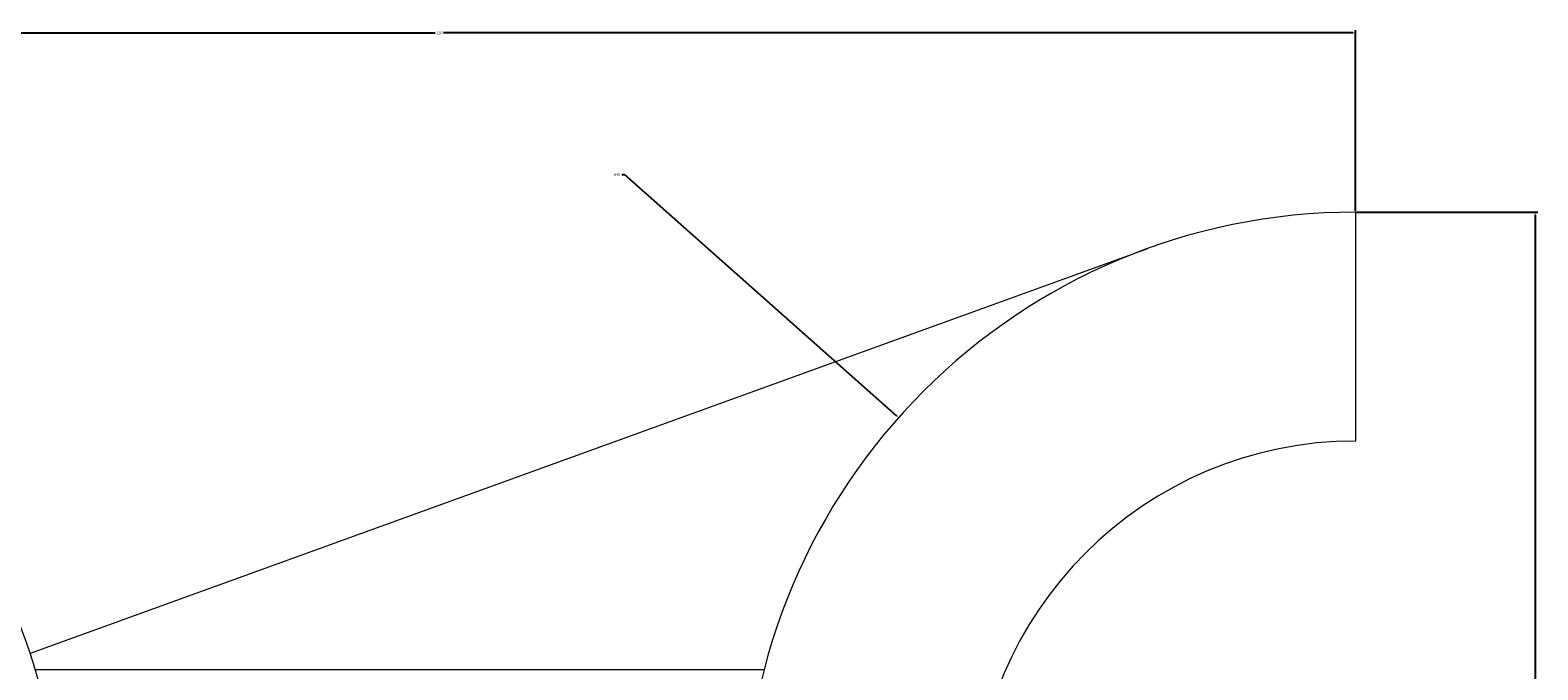
# Model space of a CAD drawing. Units: millimetres. Extents: x 3108 to 3332, y 1482 to 1586.
# Tile 5 of 5: x 3233 to 3332, y 1544 to 1586. Entities that reach past the tile are written whole.
import ezdxf

# ---------------------------------------------------------------- set-up
doc = ezdxf.new("R2010")
doc.units = ezdxf.units.MM
doc.layers.add('M-CONS', color=8, linetype='Continuous', lineweight=18)
doc.layers.add('M-DIMS', color=2, linetype='Continuous', lineweight=18)
doc.styles.get("Standard").update_dxf_attribs({"font": 'arial.ttf'})
doc.dimstyles.get("Standard").update_dxf_attribs({"dimtxt": 0.18, "dimasz": 0.18, "dimexe": 0.18, "dimexo": 0.0625, "dimgap": 0.09, "dimtad": 0, "dimtih": 1, "dimtoh": 1, "dimdec": 4, "dimzin": 0, "dimdsep": 46, "dimtxsty": 'Standard', "dimcen": 0.09, "dimadec": 0, "dimazin": 0, "dimtfac": 1, "dimtdec": 4, "dimtofl": 0, "dimtmove": 0, "dimatfit": 3, "dimfxl": 1, "dimtolj": 1, "dimtzin": 0, "dimarcsym": 0})

# ---------------------------------------------------------------- blocks, each defined once
blk = doc.blocks.new('*D2')
at = {"layer": 'Defpoints', "color": 0, "transparency": 16777216}
for p in [(3319.945, 1573.943), (3331.695, 1573.943), (3319.945, 1493.943)]:
    blk.add_point(p, dxfattribs=at)
at = {"layer": 'M-DIMS', "color": 0, "lineweight": -2, "transparency": 16777216}
for p, q in [((3320.007, 1573.943), (3331.875, 1573.943)), ((3331.695, 1573.763), (3331.695, 1534.125)), ((3331.695, 1494.123), (3331.695, 1533.761)), ((3320.007, 1493.943), (3331.875, 1493.943))]:
    blk.add_line(p, q, dxfattribs=at)
at = {"layer": 'M-DIMS', "color": 0, "transparency": 16777216}
for points in [[(3331.665, 1573.763), (3331.725, 1573.763), (3331.695, 1573.943)], [(3331.665, 1494.123), (3331.725, 1494.123), (3331.695, 1493.943)]]:
    blk.add_solid(points, dxfattribs=at)
at = {"layer": 'M-DIMS', "color": 0, "transparency": 16777216, "insert": (3331.695, 1533.943), "char_height": 0.18, "attachment_point": 5}
blk.add_mtext('\\A1;80', dxfattribs=at)
blk = doc.blocks.new('*D3')
at = {"layer": 'Defpoints', "color": 0, "transparency": 16777216}
for p in [(3319.945, 1585.693), (3319.945, 1573.943), (3199.945, 1568.943)]:
    blk.add_point(p, dxfattribs=at)
at = {"layer": 'M-DIMS', "color": 0, "lineweight": -2, "transparency": 16777216}
for p, q in [((3199.945, 1569.006), (3199.945, 1585.873)), ((3200.125, 1585.693), (3259.665, 1585.693)), ((3319.765, 1585.693), (3260.225, 1585.693)), ((3319.945, 1574.006), (3319.945, 1585.873))]:
    blk.add_line(p, q, dxfattribs=at)
at = {"layer": 'M-DIMS', "color": 0, "transparency": 16777216}
for points in [[(3200.125, 1585.723), (3200.125, 1585.663), (3199.945, 1585.693)], [(3319.765, 1585.723), (3319.765, 1585.663), (3319.945, 1585.693)]]:
    blk.add_solid(points, dxfattribs=at)
at = {"layer": 'M-DIMS', "color": 0, "transparency": 16777216, "insert": (3259.945, 1585.693), "char_height": 0.18, "attachment_point": 5}
blk.add_mtext('\\A1;120', dxfattribs=at)
blk = doc.blocks.new('*D11')
at = {"layer": 'Defpoints', "color": 0, "transparency": 16777216}
for p in [(3290.018, 1560.484), (3319.945, 1533.943)]:
    blk.add_point(p, dxfattribs=at)
at = {"layer": 'M-DIMS', "color": 0, "lineweight": -2, "transparency": 16777216}
for p, q in [((3271.882, 1576.408), (3272.062, 1576.408)), ((3272.062, 1576.408), (3289.884, 1560.603)), ((3319.855, 1533.943), (3320.035, 1533.943)), ((3319.945, 1533.853), (3319.945, 1534.033))]:
    blk.add_line(p, q, dxfattribs=at)
at = {"layer": 'M-DIMS', "color": 0, "transparency": 16777216}
blk.add_solid([(3289.904, 1560.626), (3289.864, 1560.581), (3290.018, 1560.484)], dxfattribs=at)
at = {"layer": 'M-DIMS', "color": 0, "transparency": 16777216, "insert": (3271.578, 1576.408), "char_height": 0.18, "attachment_point": 5}
blk.add_mtext('\\A1;R40', dxfattribs=at)

msp = doc.modelspace()

# ---------------------------------------------------------------- linework, layer by layer
at = {"layer": 'M-CONS'}
for p, q in [((3319.9448, 1573.9431), (3319.9448, 1558.9431)), ((3306.3058, 1571.546), (3233.1487, 1545.0111)), ((3281.2149, 1543.9431), (3233.4858, 1543.9431))]:
    msp.add_line(p, q, dxfattribs=at)
for centre, radius, start, end in [((3319.9448, 1533.9431), 40, 90, 270), ((3199.9448, 1533.9431), 35, 270, 90), ((3319.9448, 1533.9431), 25, 90, 270)]:
    msp.add_arc(centre, radius, start, end, dxfattribs=at)

# ---------------------------------------------------------------- dimensions: what is measured, and where the dimension line sits
at = {"layer": 'M-DIMS'}
dim = msp.add_linear_dim(base=(3319.9448, 1585.6931), p1=(3199.9448, 1568.9431), p2=(3319.9448, 1573.9431), dimstyle='Standard', override={"dimdec": 0, "dimlfac": 1, "dimrnd": 0, "dimzin": 0, "dimdsep": 46, "dimlunit": 2}, dxfattribs=at)
dim.commit()
dim.dimension.update_dxf_attribs({"geometry": '*D3', "text_midpoint": (3259.9448, 1585.6931)})
dim = msp.add_radius_dim(center=(3319.9448, 1533.9431), mpoint=(3290.0183, 1560.4838), dimstyle='Standard', override={"dimdec": 0, "dimlfac": 1, "dimrnd": 0, "dimzin": 0, "dimdsep": 46, "dimlunit": 2}, dxfattribs=at)
dim.commit()
dim.dimension.update_dxf_attribs({"geometry": '*D11', "text_midpoint": (3271.5777, 1576.4082), "dimtype": 164})
dim = msp.add_linear_dim(base=(3331.6948, 1573.9431), p1=(3319.9448, 1493.9431), p2=(3319.9448, 1573.9431), angle=90, dimstyle='Standard', override={"dimdec": 0, "dimlfac": 1, "dimrnd": 0, "dimzin": 0, "dimdsep": 46, "dimlunit": 2}, dxfattribs=at)
dim.commit()
dim.dimension.update_dxf_attribs({"geometry": '*D2', "text_midpoint": (3331.6948, 1533.9431)})

doc.saveas('drawing.dxf')
